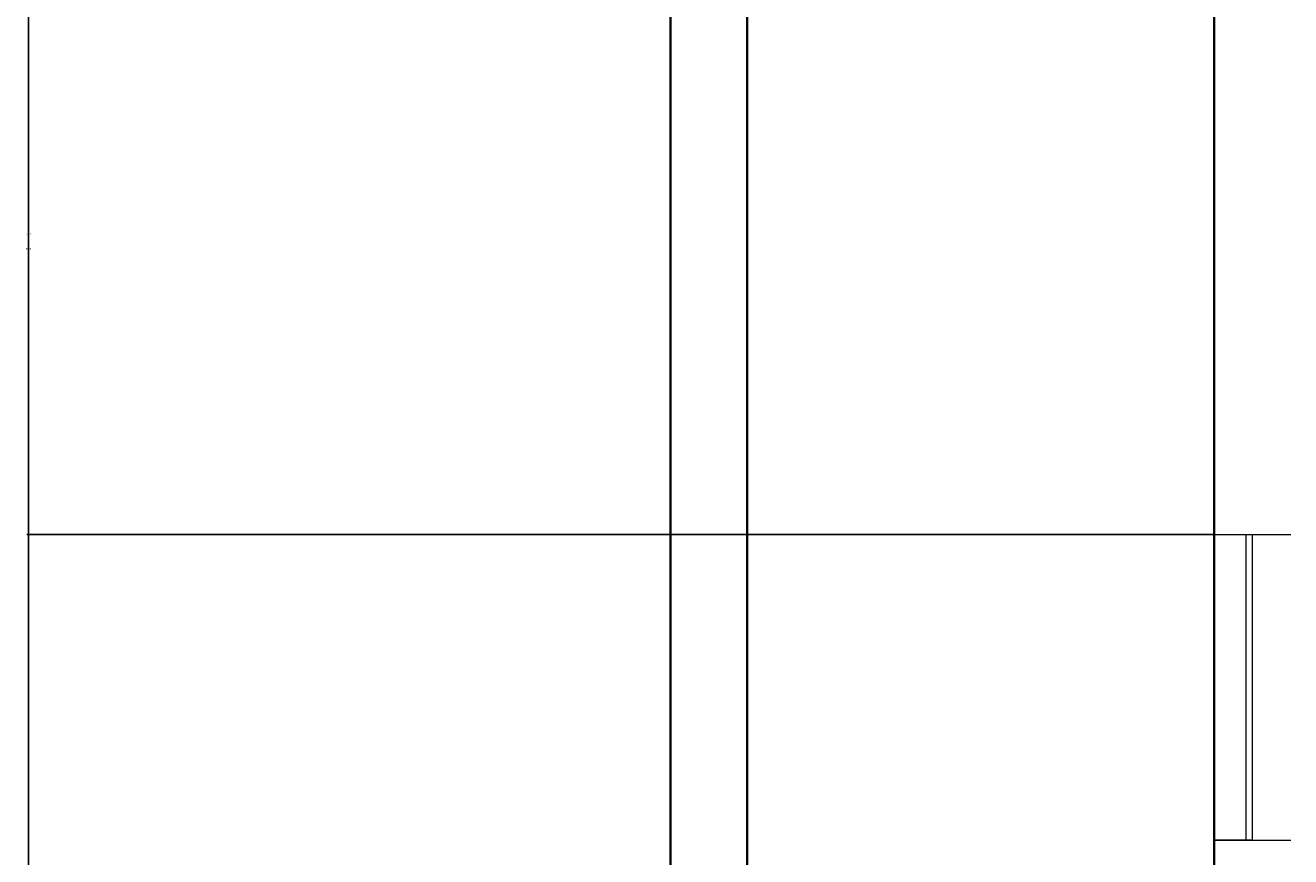
# Model space of a CAD drawing. Units: inches. Extents: x -61 to 1599, y -1316 to 257.
# Tile 44 of 204: x -61 to 88, y -380 to -282. Entities that reach past the tile are written whole.
import ezdxf

# ---------------------------------------------------------------- set-up
doc = ezdxf.new("R2010")
doc.units = ezdxf.units.IN
doc.header["$MEASUREMENT"] = 0
for name, color, linetype, lineweight in [('A-ANNO-DIMS', 2, 'Continuous', 18), ('WALLS', 4, 'Continuous', 35), ('WINDOWS', 220, 'Continuous', 18)]:
    doc.layers.add(name, color=color, linetype=linetype, lineweight=lineweight)
doc.styles.get("Standard").update_dxf_attribs({"font": 'arial.ttf'})
doc.dimstyles.get("Standard").update_dxf_attribs({"dimtxt": 0.18, "dimasz": 0.18, "dimexe": 0.18, "dimexo": 0.0625, "dimgap": 0.09, "dimtad": 0, "dimtih": 1, "dimtoh": 1, "dimdec": 0, "dimzin": 0, "dimdsep": 46, "dimlunit": 3, "dimtxsty": 'Standard', "dimcen": 0.09, "dimadec": 0, "dimazin": 0, "dimtfac": 1, "dimtdec": 0, "dimtofl": 0, "dimtmove": 0, "dimatfit": 3, "dimfxl": 1, "dimtolj": 1, "dimtzin": 0, "dimarcsym": 0})

# ---------------------------------------------------------------- blocks, each defined once
blk = doc.blocks.new('WIN-36IN')
for p, q in [((0, 4.5), (0, 9)), ((0, 9), (0, 0)), ((36, 9), (36, 0)), ((0, 5.26), (36, 5.26)), ((0, 4.5), (36, 4.5)), ((0, 4.5), (36, 4.5))]:
    blk.add_line(p, q)
blk = doc.blocks.new('*D687')
at = {"layer": 'A-ANNO-DIMS', "color": 0, "lineweight": -2, "transparency": 16777216}
for p, q in [((289.42, 181.68), (-61.08, 181.68)), ((-60.9, 181.5), (-60.9, -528.95)), ((-60.9, -1239.76), (-60.9, -529.32)), ((319.64, -1239.94), (-61.08, -1239.94))]:
    blk.add_line(p, q, dxfattribs=at)
at = {"layer": 'A-ANNO-DIMS', "color": 0, "transparency": 16777216}
for points in [[(-60.93, 181.5), (-60.87, 181.5), (-60.9, 181.68)], [(-60.93, -1239.76), (-60.87, -1239.76), (-60.9, -1239.94)]]:
    blk.add_solid(points, dxfattribs=at)
at = {"layer": 'DEFPOINTS', "color": 0, "transparency": 16777216}
for p in [(289.48, 181.68), (-60.9, -1239.94), (319.7, -1239.94)]:
    blk.add_point(p, dxfattribs=at)
at = {"layer": 'A-ANNO-DIMS', "color": 0, "transparency": 16777216, "insert": (-60.9, -529.13), "char_height": 0.18, "attachment_point": 5}
blk.add_mtext('\\A1;1421.6', dxfattribs=at)
blk = doc.blocks.new('*D691')
at = {"layer": 'A-ANNO-DIMS', "color": 0, "lineweight": -2, "transparency": 16777216}
for p, q in [((14.64, 157.68), (-61.08, 157.68)), ((-60.9, 157.5), (-60.9, -141.64)), ((-60.9, -441.14), (-60.9, -142)), ((14.64, -441.32), (-61.08, -441.32))]:
    blk.add_line(p, q, dxfattribs=at)
at = {"layer": 'A-ANNO-DIMS', "color": 0, "transparency": 16777216}
for points in [[(-60.93, 157.5), (-60.87, 157.5), (-60.9, 157.68)], [(-60.93, -441.14), (-60.87, -441.14), (-60.9, -441.32)]]:
    blk.add_solid(points, dxfattribs=at)
at = {"layer": 'DEFPOINTS', "color": 0, "transparency": 16777216}
for p in [(-60.9, 157.68), (14.7, 157.68), (14.7, -441.32)]:
    blk.add_point(p, dxfattribs=at)
at = {"layer": 'A-ANNO-DIMS', "color": 0, "transparency": 16777216, "insert": (-60.9, -141.82), "char_height": 0.18, "attachment_point": 5}
blk.add_mtext('\\A1;599', dxfattribs=at)
blk = doc.blocks.new('*D699')
at = {"layer": 'A-ANNO-DIMS', "color": 0, "lineweight": -2, "transparency": 16777216}
for p, q in [((835.64, -167.17), (-61.08, -167.17)), ((-60.9, -167.35), (-60.9, -306.73)), ((-60.9, -446.47), (-60.9, -307.09)), ((841.64, -446.65), (-61.08, -446.65))]:
    blk.add_line(p, q, dxfattribs=at)
at = {"layer": 'A-ANNO-DIMS', "color": 0, "transparency": 16777216}
for points in [[(-60.93, -167.35), (-60.87, -167.35), (-60.9, -167.17)], [(-60.93, -446.47), (-60.87, -446.47), (-60.9, -446.65)]]:
    blk.add_solid(points, dxfattribs=at)
at = {"layer": 'DEFPOINTS', "color": 0, "transparency": 16777216}
for p in [(835.7, -167.17), (-60.9, -446.65), (841.7, -446.65)]:
    blk.add_point(p, dxfattribs=at)
at = {"layer": 'A-ANNO-DIMS', "color": 0, "transparency": 16777216, "insert": (-60.9, -306.91), "char_height": 0.18, "attachment_point": 5}
blk.add_mtext('\\A1;279.5', dxfattribs=at)
blk = doc.blocks.new('*D700')
at = {"layer": 'A-ANNO-DIMS', "color": 0, "lineweight": -2, "transparency": 16777216}
for p, q in [((14.7, -616.88), (14.7, 257.46)), ((14.88, 257.28), (96.77, 257.28)), ((179.57, 257.28), (97.68, 257.28)), ((179.75, -616.88), (179.75, 257.46))]:
    blk.add_line(p, q, dxfattribs=at)
at = {"layer": 'A-ANNO-DIMS', "color": 0, "transparency": 16777216}
for points in [[(14.88, 257.31), (14.88, 257.25), (14.7, 257.28)], [(179.57, 257.31), (179.57, 257.25), (179.75, 257.28)]]:
    blk.add_solid(points, dxfattribs=at)
at = {"layer": 'DEFPOINTS', "color": 0, "transparency": 16777216}
for p in [(179.75, 257.28), (14.7, -616.94), (179.75, -616.94)]:
    blk.add_point(p, dxfattribs=at)
at = {"layer": 'A-ANNO-DIMS', "color": 0, "transparency": 16777216, "insert": (97.23, 257.28), "char_height": 0.18, "attachment_point": 5}
blk.add_mtext('\\A1;165.05', dxfattribs=at)
blk = doc.blocks.new('*D707')
at = {"layer": 'A-ANNO-DIMS', "color": 0, "lineweight": -2, "transparency": 16777216}
for p, q in [((78.64, -274.99), (-61.08, -274.99)), ((-60.9, -275.17), (-60.9, -308.47)), ((-60.9, -342.14), (-60.9, -308.84)), ((78.64, -342.32), (-61.08, -342.32))]:
    blk.add_line(p, q, dxfattribs=at)
at = {"layer": 'A-ANNO-DIMS', "color": 0, "transparency": 16777216}
for points in [[(-60.93, -275.17), (-60.87, -275.17), (-60.9, -274.99)], [(-60.93, -342.14), (-60.87, -342.14), (-60.9, -342.32)]]:
    blk.add_solid(points, dxfattribs=at)
at = {"layer": 'DEFPOINTS', "color": 0, "transparency": 16777216}
for p in [(78.7, -274.99), (-60.9, -342.32), (78.7, -342.32)]:
    blk.add_point(p, dxfattribs=at)
at = {"layer": 'A-ANNO-DIMS', "color": 0, "transparency": 16777216, "insert": (-60.9, -308.66), "char_height": 0.18, "attachment_point": 5}
blk.add_mtext('\\A1;67.33', dxfattribs=at)

msp = doc.modelspace()

# ---------------------------------------------------------------- linework, layer by layer
at = {"layer": 'WALLS'}
for p, q in [((14.7028, 157.6771), (14.7028, -441.3229)), ((23.7028, -175.3229), (23.7028, -432.3229)), ((78.7028, -175.3229), (78.7028, -432.3229))]:
    msp.add_line(p, q, dxfattribs=at)

# ---------------------------------------------------------------- block references
at = {"layer": 'WINDOWS', "rotation": 90.00000000000006}
msp.add_blockref('WIN-36IN', (87.7029, -378.3189), dxfattribs=at)

# ---------------------------------------------------------------- dimensions: what is measured, and where the dimension line sits
at = {"layer": 'A-ANNO-DIMS'}
dim = msp.add_linear_dim(base=(179.7521, 257.2771), p1=(14.7028, -616.9446), p2=(179.7521, -616.9446), dimstyle='Standard', override={"dimdec": 2, "dimlfac": 1, "dimrnd": 0, "dimzin": 0, "dimdsep": 46, "dimlunit": 2}, dxfattribs=at)
dim.commit()
dim.dimension.update_dxf_attribs({"geometry": '*D700', "text_midpoint": (97.2274, 257.2771)})
for base, p1, p2, override, picture, middle in [((-60.8972, -1239.9446), (289.4807, 181.6771), (319.7028, -1239.9446), {"dimdec": 1, "dimlfac": 1, "dimrnd": 0, "dimzin": 0, "dimdsep": 46, "dimlunit": 2}, '*D687', (-60.8972, -529.1337)), ((-60.8972, 157.6771), (14.7028, -441.3229), (14.7028, 157.6771), {"dimdec": 0, "dimlfac": 1, "dimrnd": 0, "dimzin": 0, "dimdsep": 46, "dimlunit": 2}, '*D691', (-60.8972, -141.8229)), ((-60.8972, -446.6462), (835.7028, -167.169), (841.7028, -446.6462), {"dimdec": 1, "dimlfac": 1, "dimrnd": 0, "dimzin": 0, "dimdsep": 46, "dimlunit": 2}, '*D699', (-60.8972, -306.9076)), ((-60.8972, -342.3189), (78.7028, -274.9938), (78.7028, -342.3189), {"dimdec": 2, "dimlfac": 1, "dimrnd": 0, "dimzin": 0, "dimdsep": 46, "dimlunit": 2}, '*D707', (-60.8972, -308.6563))]:
    dim = msp.add_linear_dim(base=base, p1=p1, p2=p2, angle=90, dimstyle='Standard', override=override, dxfattribs=at)
    dim.commit()
    dim.dimension.update_dxf_attribs({"geometry": picture, "text_midpoint": middle})

doc.saveas('drawing.dxf')
